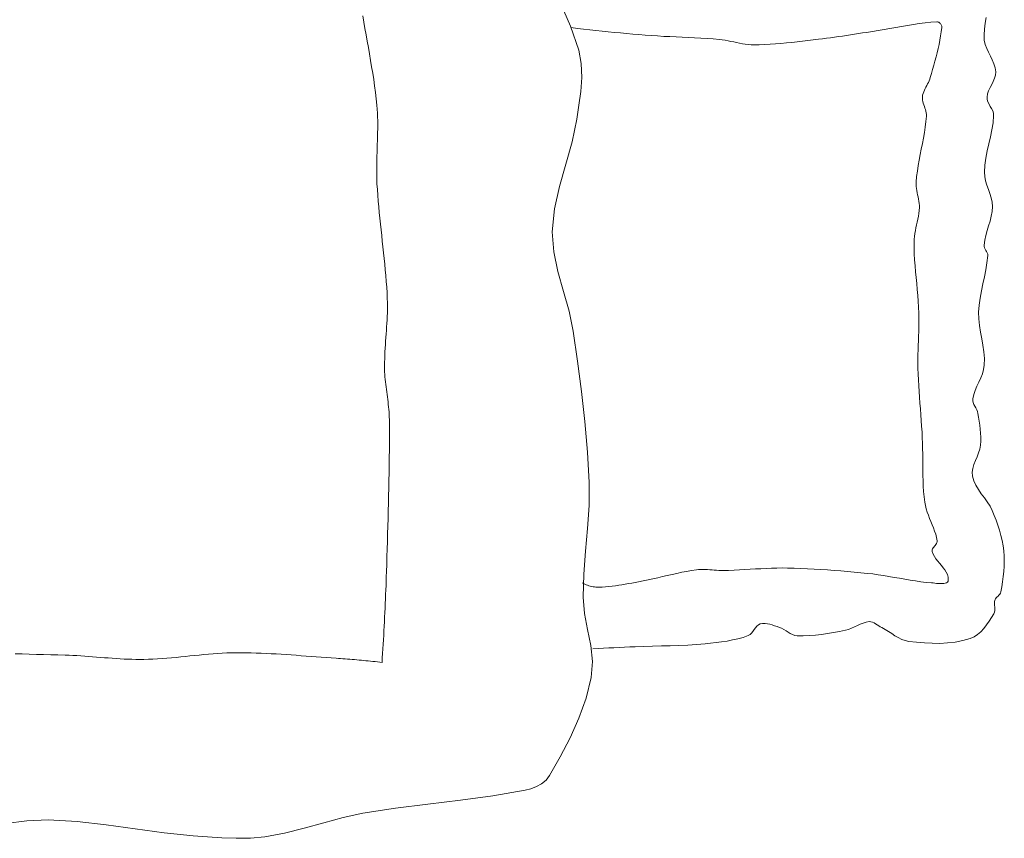
# Model space of a CAD drawing. Units: inches. Extents: x -36302355 to 648, y -221479757 to 75.
# Tile 18 of 37: x 555 to 590, y -530 to -501. Entities that reach past the tile are written whole.
import ezdxf

# ---------------------------------------------------------------- set-up
doc = ezdxf.new("R2010")
doc.units = ezdxf.units.IN
doc.header["$MEASUREMENT"] = 0
doc.layers.add('A-FURN', color=8, linetype='Continuous', lineweight=13)

# ---------------------------------------------------------------- blocks, each defined once
blk = doc.blocks.new('BED-DOUBLE')
for p, q in [((46.094, 79.977), (45.912, 79.943)), ((46.276, 80.001), (46.094, 79.977)), ((46.457, 80.015), (46.276, 80.001)), ((46.638, 80.019), (46.457, 80.015)), ((46.819, 80.013), (46.638, 80.019)), ((47.001, 80.001), (46.819, 80.013)), ((47.182, 79.981), (47.001, 80.001)), ((47.363, 79.957), (47.182, 79.981)), ((29.156, 79.653), (29.019, 79.595)), ((29.295, 79.695), (29.156, 79.653)), ((29.439, 79.716), (29.295, 79.695)), ((29.555, 79.707), (29.439, 79.716)), ((29.667, 79.676), (29.555, 79.707)), ((29.776, 79.63), (29.667, 79.676)), ((29.885, 79.575), (29.776, 79.63)), ((30.892, 79.636), (30.811, 79.61)), ((30.976, 79.644), (30.892, 79.636)), ((31.228, 79.624), (30.976, 79.644)), ((31.477, 79.585), (31.228, 79.624)), ((45.03, 79.665), (44.859, 79.595)), ((45.203, 79.731), (45.03, 79.665)), ((45.378, 79.793), (45.203, 79.731)), ((45.554, 79.85), (45.378, 79.793)), ((45.733, 79.9), (45.554, 79.85)), ((45.912, 79.943), (45.733, 79.9)), ((47.542, 79.928), (47.363, 79.957)), ((47.721, 79.897), (47.542, 79.928)), ((47.762, 79.883), (47.721, 79.897)), ((47.799, 79.86), (47.762, 79.883)), ((47.832, 79.831), (47.799, 79.86)), ((47.865, 79.797), (47.832, 79.831)), ((47.897, 79.763), (47.865, 79.797)), ((47.93, 79.732), (47.897, 79.763)), ((47.966, 79.705), (47.93, 79.732)), ((48.005, 79.687), (47.966, 79.705)), ((48.065, 79.675), (48.005, 79.687)), ((48.126, 79.673), (48.065, 79.675)), ((48.189, 79.677), (48.126, 79.673)), ((48.253, 79.684), (48.189, 79.677)), ((48.316, 79.688), (48.253, 79.684)), ((48.376, 79.687), (48.316, 79.688)), ((48.434, 79.676), (48.376, 79.687)), ((48.487, 79.652), (48.434, 79.676)), ((48.617, 79.57), (48.487, 79.652)), ((27.733, 79.348), (27.532, 79.381)), ((27.935, 79.319), (27.733, 79.348)), ((28.135, 79.305), (27.935, 79.319)), ((28.332, 79.316), (28.135, 79.305)), ((28.475, 79.348), (28.332, 79.316)), ((28.614, 79.399), (28.475, 79.348)), ((28.75, 79.461), (28.614, 79.399)), ((28.885, 79.529), (28.75, 79.461)), ((29.019, 79.595), (28.885, 79.529)), ((29.994, 79.518), (29.885, 79.575)), ((30.103, 79.467), (29.994, 79.518)), ((30.215, 79.429), (30.103, 79.467)), ((30.331, 79.412), (30.215, 79.429)), ((30.415, 79.419), (30.331, 79.412)), ((30.496, 79.445), (30.415, 79.419)), ((30.575, 79.483), (30.496, 79.445)), ((30.654, 79.527), (30.575, 79.483)), ((30.732, 79.571), (30.654, 79.527)), ((30.811, 79.61), (30.732, 79.571)), ((31.725, 79.534), (31.477, 79.585)), ((31.973, 79.478), (31.725, 79.534)), ((32.221, 79.421), (31.973, 79.478)), ((32.469, 79.372), (32.221, 79.421)), ((32.718, 79.336), (32.469, 79.372)), ((32.97, 79.321), (32.718, 79.336)), ((33.123, 79.331), (32.97, 79.321)), ((33.273, 79.362), (33.123, 79.331)), ((33.423, 79.406), (33.273, 79.362)), ((33.571, 79.458), (33.423, 79.406)), ((33.72, 79.51), (33.571, 79.458)), ((33.869, 79.555), (33.72, 79.51)), ((34.02, 79.587), (33.869, 79.555)), ((34.173, 79.598), (34.02, 79.587)), ((34.345, 79.587), (34.173, 79.598)), ((34.515, 79.557), (34.345, 79.587)), ((34.684, 79.516), (34.515, 79.557)), ((34.852, 79.467), (34.684, 79.516)), ((35.02, 79.416), (34.852, 79.467)), ((35.188, 79.369), (35.02, 79.416)), ((35.358, 79.33), (35.188, 79.369)), ((35.529, 79.305), (35.358, 79.33)), ((35.577, 79.308), (35.529, 79.305)), ((35.623, 79.323), (35.577, 79.308)), ((35.669, 79.345), (35.623, 79.323)), ((35.714, 79.371), (35.669, 79.345)), ((35.758, 79.398), (35.714, 79.371)), ((35.804, 79.42), (35.758, 79.398)), ((35.85, 79.435), (35.804, 79.42)), ((35.898, 79.439), (35.85, 79.435)), ((36.149, 79.41), (35.898, 79.439)), ((36.398, 79.368), (36.149, 79.41)), ((36.646, 79.318), (36.398, 79.368)), ((36.894, 79.264), (36.646, 79.318)), ((39.283, 79.299), (39.051, 79.265)), ((39.515, 79.318), (39.283, 79.299)), ((39.748, 79.315), (39.515, 79.318)), ((39.902, 79.292), (39.748, 79.315)), ((40.051, 79.248), (39.902, 79.292)), ((44.409, 79.317), (44.266, 79.21)), ((44.554, 79.421), (44.409, 79.317)), ((44.703, 79.516), (44.554, 79.421)), ((44.859, 79.595), (44.703, 79.516)), ((48.749, 79.484), (48.617, 79.57)), ((48.879, 79.394), (48.749, 79.484)), ((49.004, 79.298), (48.879, 79.394)), ((49.119, 79.194), (49.004, 79.298)), ((37.142, 79.212), (36.894, 79.264)), ((37.39, 79.167), (37.142, 79.212)), ((37.64, 79.133), (37.39, 79.167)), ((37.891, 79.115), (37.64, 79.133)), ((38.124, 79.119), (37.891, 79.115)), ((38.357, 79.144), (38.124, 79.119)), ((38.588, 79.18), (38.357, 79.144)), ((38.82, 79.223), (38.588, 79.18)), ((39.051, 79.265), (38.82, 79.223)), ((40.198, 79.189), (40.051, 79.248)), ((40.343, 79.122), (40.198, 79.189)), ((40.488, 79.055), (40.343, 79.122)), ((40.634, 78.992), (40.488, 79.055)), ((40.783, 78.942), (40.634, 78.992)), ((40.936, 78.91), (40.783, 78.942)), ((41.066, 78.924), (41.002, 78.91)), ((41.128, 78.95), (41.066, 78.924)), ((41.19, 78.981), (41.128, 78.95)), ((41.252, 79.016), (41.19, 78.981)), ((41.315, 79.048), (41.252, 79.016)), ((41.378, 79.075), (41.315, 79.048)), ((41.444, 79.093), (41.378, 79.075)), ((41.582, 79.116), (41.444, 79.093)), ((41.721, 79.137), (41.582, 79.116)), ((41.86, 79.157), (41.721, 79.137)), ((42, 79.173), (41.86, 79.157)), ((42.139, 79.184), (42, 79.173)), ((42.279, 79.19), (42.139, 79.184)), ((42.419, 79.19), (42.279, 79.19)), ((42.558, 79.182), (42.419, 79.19)), ((42.698, 79.158), (42.558, 79.182)), ((42.835, 79.114), (42.698, 79.158)), ((42.971, 79.06), (42.835, 79.114)), ((43.106, 79.003), (42.971, 79.06)), ((43.241, 78.95), (43.106, 79.003)), ((43.377, 78.91), (43.241, 78.95)), ((43.817, 78.944), (43.651, 78.898)), ((43.972, 79.016), (43.817, 78.944)), ((44.121, 79.107), (43.972, 79.016)), ((44.266, 79.21), (44.121, 79.107)), ((49.219, 79.081), (49.119, 79.194)), ((49.301, 78.957), (49.219, 79.081)), ((49.36, 78.82), (49.301, 78.957)), ((41.002, 78.91), (40.936, 78.91)), ((43.513, 78.89), (43.377, 78.91)), ((43.651, 78.898), (43.513, 78.89)), ((49.432, 78.561), (49.36, 78.82)), ((49.482, 78.296), (49.432, 78.561)), ((49.513, 78.027), (49.482, 78.296)), ((46.868, 77.87), (46.947, 77.928)), ((46.947, 77.928), (47.028, 77.978)), ((47.028, 77.978), (47.112, 78.016)), ((47.112, 78.016), (47.2, 78.041)), ((47.2, 78.041), (47.293, 78.049)), ((47.293, 78.049), (47.337, 78.04)), ((47.337, 78.04), (47.371, 78.018)), ((47.371, 78.018), (47.396, 77.983)), ((47.396, 77.983), (47.413, 77.939)), ((47.413, 77.939), (47.423, 77.887)), ((47.423, 77.887), (47.427, 77.828)), ((49.527, 77.755), (49.513, 78.027)), ((27.683, 77.649), (27.684, 77.671)), ((27.699, 77.441), (27.683, 77.649)), ((27.684, 77.671), (27.689, 77.693)), ((27.689, 77.693), (27.699, 77.715)), ((27.699, 77.715), (27.712, 77.735)), ((27.712, 77.735), (27.728, 77.755)), ((27.728, 77.755), (27.746, 77.773)), ((27.746, 77.773), (27.767, 77.789)), ((27.767, 77.789), (27.789, 77.803)), ((27.789, 77.803), (27.812, 77.813)), ((27.812, 77.813), (27.835, 77.821)), ((27.835, 77.821), (27.858, 77.824)), ((27.858, 77.824), (27.88, 77.824)), ((27.88, 77.824), (28.029, 77.804)), ((28.029, 77.804), (28.178, 77.781)), ((28.178, 77.781), (28.326, 77.754)), ((28.326, 77.754), (28.474, 77.723)), ((28.474, 77.723), (28.621, 77.691)), ((28.621, 77.691), (28.768, 77.655)), ((28.768, 77.655), (28.915, 77.618)), ((28.915, 77.618), (29.061, 77.58)), ((29.061, 77.58), (29.206, 77.54)), ((29.206, 77.54), (29.352, 77.499)), ((45.467, 77.529), (45.579, 77.57)), ((45.579, 77.57), (45.692, 77.607)), ((45.692, 77.607), (45.806, 77.636)), ((45.806, 77.636), (45.922, 77.659)), ((45.922, 77.659), (45.956, 77.659)), ((45.956, 77.659), (45.988, 77.65)), ((45.988, 77.65), (46.02, 77.634)), ((46.02, 77.634), (46.051, 77.613)), ((46.051, 77.613), (46.082, 77.589)), ((46.082, 77.589), (46.112, 77.564)), ((46.112, 77.564), (46.142, 77.538)), ((46.142, 77.538), (46.172, 77.515)), ((46.388, 77.515), (46.473, 77.56)), ((46.473, 77.56), (46.555, 77.615)), ((46.555, 77.615), (46.635, 77.677)), ((46.635, 77.677), (46.713, 77.741)), ((46.713, 77.741), (46.79, 77.807)), ((46.79, 77.807), (46.868, 77.87)), ((47.412, 77.574), (47.405, 77.515)), ((47.418, 77.637), (47.412, 77.574)), ((47.424, 77.701), (47.418, 77.637)), ((47.427, 77.766), (47.424, 77.701)), ((47.427, 77.828), (47.427, 77.766)), ((49.526, 77.481), (49.527, 77.755)), ((27.721, 77.234), (27.699, 77.441)), ((27.746, 77.027), (27.721, 77.234)), ((29.352, 77.499), (29.497, 77.458)), ((29.497, 77.458), (29.643, 77.417)), ((29.643, 77.417), (29.7, 77.398)), ((29.7, 77.398), (29.757, 77.376)), ((29.757, 77.376), (29.813, 77.349)), ((29.813, 77.349), (29.867, 77.321)), ((29.867, 77.321), (29.922, 77.292)), ((29.922, 77.292), (29.977, 77.263)), ((29.977, 77.263), (30.031, 77.234)), ((30.031, 77.234), (30.086, 77.207)), ((30.086, 77.207), (30.142, 77.184)), ((30.599, 77.187), (30.656, 77.207)), ((30.656, 77.207), (30.712, 77.227)), ((30.712, 77.227), (30.768, 77.246)), ((30.768, 77.246), (30.824, 77.261)), ((30.824, 77.261), (30.881, 77.273)), ((30.881, 77.273), (30.938, 77.28)), ((30.938, 77.28), (30.995, 77.28)), ((30.995, 77.28), (31.19, 77.261)), ((31.19, 77.261), (31.384, 77.237)), ((31.384, 77.237), (31.577, 77.207)), ((31.577, 77.207), (31.77, 77.173)), ((44.193, 77.181), (44.381, 77.199)), ((44.381, 77.199), (44.568, 77.222)), ((44.568, 77.222), (44.684, 77.244)), ((44.684, 77.244), (44.799, 77.273)), ((44.799, 77.273), (44.912, 77.309)), ((44.912, 77.309), (45.023, 77.35)), ((45.023, 77.35), (45.135, 77.394)), ((45.135, 77.394), (45.245, 77.439)), ((45.245, 77.439), (45.356, 77.485)), ((45.356, 77.485), (45.467, 77.529)), ((46.172, 77.515), (46.203, 77.496)), ((46.203, 77.496), (46.234, 77.483)), ((46.234, 77.483), (46.266, 77.478)), ((46.266, 77.478), (46.299, 77.482)), ((46.299, 77.482), (46.388, 77.515)), ((47.383, 77.273), (47.36, 77.084)), ((47.4, 77.462), (47.383, 77.273)), ((47.405, 77.515), (47.4, 77.462)), ((49.49, 76.936), (49.513, 77.208)), ((49.513, 77.208), (49.526, 77.481)), ((27.776, 76.821), (27.746, 77.027)), ((30.142, 77.184), (30.199, 77.164)), ((30.199, 77.164), (30.257, 77.148)), ((30.257, 77.148), (30.316, 77.139)), ((30.316, 77.139), (30.374, 77.137)), ((30.374, 77.137), (30.43, 77.142)), ((30.43, 77.142), (30.487, 77.153)), ((30.487, 77.153), (30.543, 77.169)), ((30.543, 77.169), (30.599, 77.187)), ((31.77, 77.173), (31.963, 77.137)), ((31.963, 77.137), (32.155, 77.099)), ((32.155, 77.099), (32.348, 77.062)), ((32.348, 77.062), (32.54, 77.025)), ((32.54, 77.025), (32.733, 76.991)), ((32.733, 76.991), (32.927, 76.961)), ((32.927, 76.961), (33.12, 76.936)), ((33.12, 76.936), (33.315, 76.917)), ((33.315, 76.917), (33.39, 76.915)), ((33.39, 76.915), (33.465, 76.919)), ((33.465, 76.919), (33.54, 76.927)), ((33.54, 76.927), (33.614, 76.939)), ((33.614, 76.939), (33.689, 76.954)), ((33.689, 76.954), (33.763, 76.97)), ((33.763, 76.97), (33.838, 76.986)), ((33.838, 76.986), (33.912, 77.002)), ((33.912, 77.002), (33.987, 77.015)), ((33.987, 77.015), (34.062, 77.026)), ((34.062, 77.026), (34.137, 77.032)), ((34.137, 77.032), (34.212, 77.032)), ((34.212, 77.032), (34.314, 77.026)), ((34.314, 77.026), (34.416, 77.014)), ((34.416, 77.014), (34.517, 76.997)), ((34.517, 76.997), (34.618, 76.978)), ((34.618, 76.978), (34.718, 76.956)), ((34.718, 76.956), (34.819, 76.934)), ((34.819, 76.934), (34.92, 76.912)), ((34.92, 76.912), (35.02, 76.891)), ((35.02, 76.891), (35.121, 76.873)), ((35.121, 76.873), (35.223, 76.858)), ((35.223, 76.858), (35.324, 76.848)), ((35.324, 76.848), (35.426, 76.845)), ((35.426, 76.845), (35.634, 76.847)), ((35.634, 76.847), (35.842, 76.854)), ((35.842, 76.854), (36.05, 76.866)), ((36.05, 76.866), (36.258, 76.881)), ((36.258, 76.881), (36.465, 76.899)), ((36.465, 76.899), (36.673, 76.918)), ((36.673, 76.918), (36.88, 76.938)), ((36.88, 76.938), (37.088, 76.957)), ((37.088, 76.957), (37.296, 76.976)), ((37.296, 76.976), (37.503, 76.992)), ((37.503, 76.992), (37.711, 77.005)), ((37.711, 77.005), (37.919, 77.014)), ((37.919, 77.014), (38.081, 77.017)), ((38.081, 77.017), (38.242, 77.017)), ((38.242, 77.017), (38.404, 77.015)), ((38.404, 77.015), (38.566, 77.011)), ((38.566, 77.011), (38.727, 77.006)), ((38.727, 77.006), (38.889, 77)), ((38.889, 77), (39.051, 76.993)), ((39.051, 76.993), (39.212, 76.988)), ((39.212, 76.988), (39.374, 76.984)), ((39.374, 76.984), (39.536, 76.981)), ((39.536, 76.981), (39.697, 76.981)), ((39.697, 76.981), (39.859, 76.984)), ((39.859, 76.984), (40.063, 76.991)), ((40.063, 76.991), (40.267, 77)), ((40.267, 77), (40.471, 77.011)), ((40.471, 77.011), (40.675, 77.024)), ((40.675, 77.024), (40.879, 77.038)), ((40.879, 77.038), (41.082, 77.053)), ((41.082, 77.053), (41.286, 77.068)), ((41.286, 77.068), (41.49, 77.083)), ((41.49, 77.083), (41.694, 77.098)), ((41.694, 77.098), (41.898, 77.112)), ((41.898, 77.112), (42.102, 77.125)), ((42.102, 77.125), (42.306, 77.136)), ((42.306, 77.136), (42.494, 77.144)), ((42.494, 77.144), (42.683, 77.148)), ((42.683, 77.148), (42.872, 77.151)), ((42.872, 77.151), (43.061, 77.152)), ((43.061, 77.152), (43.25, 77.152)), ((43.25, 77.152), (43.439, 77.153)), ((43.439, 77.153), (43.628, 77.156)), ((43.628, 77.156), (43.817, 77.161)), ((43.817, 77.161), (44.005, 77.169)), ((44.005, 77.169), (44.193, 77.181)), ((47.334, 76.896), (47.305, 76.708)), ((47.36, 77.084), (47.334, 76.896)), ((49.459, 76.667), (49.49, 76.936)), ((27.808, 76.615), (27.776, 76.821)), ((27.843, 76.41), (27.808, 76.615)), ((47.273, 76.52), (47.241, 76.333)), ((47.305, 76.708), (47.273, 76.52)), ((49.387, 76.412), (49.432, 76.537)), ((49.432, 76.537), (49.459, 76.667)), ((27.879, 76.204), (27.843, 76.41)), ((27.915, 75.999), (27.879, 76.204)), ((47.241, 76.333), (47.208, 76.145)), ((49.184, 76.059), (49.258, 76.175)), ((49.258, 76.175), (49.327, 76.292)), ((49.327, 76.292), (49.387, 76.412)), ((27.952, 75.793), (27.915, 75.999)), ((47.175, 75.958), (47.144, 75.77)), ((47.208, 76.145), (47.175, 75.958)), ((48.971, 75.709), (49.036, 75.827)), ((49.036, 75.827), (49.108, 75.944)), ((49.108, 75.944), (49.184, 76.059)), ((27.987, 75.588), (27.952, 75.793)), ((28.021, 75.382), (27.987, 75.588)), ((47.115, 75.582), (47.089, 75.394)), ((47.144, 75.77), (47.115, 75.582)), ((48.806, 75.441), (48.836, 75.495)), ((48.836, 75.495), (48.871, 75.549)), ((48.871, 75.549), (48.907, 75.602)), ((48.907, 75.602), (48.941, 75.655)), ((48.941, 75.655), (48.971, 75.709)), ((28.053, 75.176), (28.021, 75.382)), ((28.074, 75.036), (28.053, 75.176)), ((47.068, 75.205), (47.044, 74.972)), ((47.089, 75.394), (47.068, 75.205)), ((48.764, 75.269), (48.767, 75.329)), ((48.781, 75.161), (48.764, 75.269)), ((48.767, 75.329), (48.782, 75.386)), ((48.812, 75.056), (48.781, 75.161)), ((48.782, 75.386), (48.806, 75.441)), ((28.095, 74.896), (28.074, 75.036)), ((28.117, 74.755), (28.095, 74.896)), ((47.044, 74.972), (47.022, 74.739)), ((48.854, 74.954), (48.812, 75.056)), ((48.901, 74.853), (48.854, 74.954)), ((48.95, 74.751), (48.901, 74.853)), ((28.139, 74.615), (28.117, 74.755)), ((28.161, 74.475), (28.139, 74.615)), ((28.182, 74.335), (28.161, 74.475)), ((47.001, 74.505), (46.981, 74.272)), ((47.022, 74.739), (47.001, 74.505)), ((48.996, 74.649), (48.95, 74.751)), ((49.036, 74.546), (48.996, 74.649)), ((49.064, 74.439), (49.036, 74.546)), ((49.105, 74.229), (49.064, 74.439)), ((28.203, 74.194), (28.182, 74.335)), ((28.224, 74.054), (28.203, 74.194)), ((46.981, 74.272), (46.962, 74.038)), ((49.144, 74.017), (49.105, 74.229)), ((28.243, 73.914), (28.224, 74.054)), ((28.262, 73.773), (28.243, 73.914)), ((28.279, 73.632), (28.262, 73.773)), ((46.945, 73.805), (46.929, 73.571)), ((46.962, 74.038), (46.945, 73.805)), ((49.181, 73.805), (49.144, 74.017)), ((49.212, 73.592), (49.181, 73.805)), ((28.296, 73.491), (28.279, 73.632)), ((28.317, 73.302), (28.296, 73.491)), ((46.929, 73.571), (46.916, 73.337)), ((49.238, 73.379), (49.212, 73.592)), ((28.339, 73.113), (28.317, 73.302)), ((28.361, 72.924), (28.339, 73.113)), ((46.904, 73.103), (46.894, 72.869)), ((46.916, 73.337), (46.904, 73.103)), ((49.255, 73.166), (49.238, 73.379)), ((49.263, 72.952), (49.255, 73.166)), ((28.383, 72.734), (28.361, 72.924)), ((28.404, 72.545), (28.383, 72.734)), ((46.894, 72.869), (46.886, 72.635)), ((49.248, 72.654), (49.26, 72.738)), ((49.26, 72.738), (49.263, 72.952)), ((28.424, 72.356), (28.404, 72.545)), ((28.442, 72.166), (28.424, 72.356)), ((46.88, 72.401), (46.878, 72.212)), ((46.886, 72.635), (46.88, 72.401)), ((49.04, 72.269), (49.087, 72.345)), ((49.087, 72.345), (49.136, 72.42)), ((49.136, 72.42), (49.181, 72.496)), ((49.181, 72.496), (49.22, 72.573)), ((49.22, 72.573), (49.248, 72.654)), ((28.458, 71.976), (28.442, 72.166)), ((46.878, 72.212), (46.88, 72.024)), ((46.88, 72.024), (46.885, 71.835)), ((48.909, 71.945), (48.938, 72.028)), ((48.938, 72.028), (48.965, 72.11)), ((48.965, 72.11), (48.998, 72.191)), ((48.998, 72.191), (49.04, 72.269)), ((28.471, 71.786), (28.458, 71.976)), ((28.482, 71.596), (28.471, 71.786)), ((46.885, 71.835), (46.892, 71.647)), ((48.827, 71.607), (48.837, 71.692)), ((48.837, 71.692), (48.856, 71.777)), ((48.856, 71.777), (48.88, 71.861)), ((48.88, 71.861), (48.909, 71.945)), ((28.488, 71.406), (28.482, 71.596)), ((28.491, 71.216), (28.488, 71.406)), ((46.892, 71.647), (46.902, 71.458)), ((46.902, 71.458), (46.912, 71.27)), ((48.828, 71.523), (48.827, 71.607)), ((48.842, 71.44), (48.828, 71.523)), ((48.872, 71.375), (48.842, 71.44)), ((48.919, 71.32), (48.872, 71.375)), ((48.978, 71.271), (48.919, 71.32)), ((28.467, 70.911), (28.48, 71.012)), ((28.48, 71.012), (28.488, 71.114)), ((28.488, 71.114), (28.491, 71.216)), ((46.912, 71.27), (46.923, 71.081)), ((46.923, 71.081), (46.934, 70.893)), ((49.043, 71.226), (48.978, 71.271)), ((49.109, 71.182), (49.043, 71.226)), ((49.17, 71.134), (49.109, 71.182)), ((49.221, 71.08), (49.17, 71.134)), ((49.256, 71.016), (49.221, 71.08)), ((49.316, 70.833), (49.256, 71.016)), ((28.411, 70.608), (28.432, 70.709)), ((28.432, 70.709), (28.451, 70.81)), ((28.451, 70.81), (28.467, 70.911)), ((46.934, 70.893), (46.944, 70.704)), ((46.944, 70.704), (46.954, 70.516)), ((49.367, 70.648), (49.316, 70.833)), ((49.409, 70.46), (49.367, 70.648)), ((28.33, 70.205), (28.348, 70.306)), ((28.348, 70.306), (28.368, 70.407)), ((28.368, 70.407), (28.389, 70.508)), ((28.389, 70.508), (28.411, 70.608)), ((46.954, 70.516), (46.961, 70.327)), ((46.961, 70.327), (46.966, 70.138)), ((49.445, 70.27), (49.409, 70.46)), ((49.474, 70.079), (49.445, 70.27)), ((28.285, 69.785), (28.303, 70.002)), ((28.303, 70.002), (28.315, 70.104)), ((28.315, 70.104), (28.33, 70.205)), ((46.964, 69.98), (46.959, 69.901)), ((46.966, 70.059), (46.964, 69.98)), ((46.966, 70.138), (46.966, 70.059)), ((49.499, 69.887), (49.474, 70.079)), ((28.27, 69.568), (28.285, 69.785)), ((46.936, 69.585), (46.932, 69.506)), ((46.941, 69.664), (46.936, 69.585)), ((46.947, 69.743), (46.941, 69.664)), ((46.954, 69.822), (46.947, 69.743)), ((46.959, 69.901), (46.954, 69.822)), ((49.521, 69.695), (49.499, 69.887)), ((49.541, 69.503), (49.521, 69.695)), ((28.244, 69.133), (28.256, 69.35)), ((28.256, 69.35), (28.27, 69.568)), ((46.932, 69.506), (46.93, 69.427)), ((46.93, 69.427), (46.93, 69.349)), ((46.93, 69.349), (46.934, 69.27)), ((46.934, 69.27), (46.943, 69.192)), ((49.567, 69.196), (49.541, 69.503)), ((28.223, 68.697), (28.234, 68.915)), ((28.234, 68.915), (28.244, 69.133)), ((46.943, 69.192), (46.968, 69.02)), ((46.968, 69.02), (46.997, 68.85)), ((49.586, 68.889), (49.567, 69.196)), ((49.6, 68.581), (49.586, 68.889)), ((28.213, 68.48), (28.223, 68.697)), ((46.997, 68.85), (47.03, 68.679)), ((47.03, 68.679), (47.066, 68.51)), ((49.611, 68.273), (49.6, 68.581)), ((28.192, 68.045), (28.203, 68.262)), ((28.203, 68.262), (28.213, 68.48)), ((47.066, 68.51), (47.103, 68.34)), ((47.103, 68.34), (47.142, 68.171)), ((49.619, 67.964), (49.611, 68.273)), ((28.18, 67.827), (28.192, 68.045)), ((47.142, 68.171), (47.182, 68.002)), ((47.182, 68.002), (47.221, 67.833)), ((49.627, 67.656), (49.619, 67.964)), ((28.15, 67.392), (28.166, 67.61)), ((28.166, 67.61), (28.18, 67.827)), ((47.221, 67.833), (47.26, 67.664)), ((47.26, 67.664), (47.297, 67.495)), ((49.636, 67.348), (49.627, 67.656)), ((28.113, 66.959), (28.132, 67.176)), ((28.132, 67.176), (28.15, 67.392)), ((47.297, 67.495), (47.332, 67.325)), ((47.332, 67.325), (47.364, 67.155)), ((47.364, 67.155), (47.385, 67.039)), ((49.647, 67.04), (49.636, 67.348)), ((28.094, 66.742), (28.113, 66.959)), ((47.385, 67.039), (47.406, 66.924)), ((47.406, 66.924), (47.428, 66.809)), ((47.428, 66.809), (47.448, 66.693)), ((49.655, 66.854), (49.647, 67.04)), ((49.664, 66.668), (49.655, 66.854)), ((28.053, 66.309), (28.074, 66.526)), ((28.074, 66.526), (28.094, 66.742)), ((47.448, 66.693), (47.468, 66.577)), ((47.468, 66.577), (47.487, 66.462)), ((47.487, 66.462), (47.504, 66.346)), ((49.672, 66.482), (49.664, 66.668)), ((49.68, 66.296), (49.672, 66.482)), ((28.032, 66.093), (28.053, 66.309)), ((47.504, 66.346), (47.519, 66.23)), ((47.519, 66.23), (47.532, 66.113)), ((47.532, 66.113), (47.543, 65.997)), ((49.689, 66.11), (49.68, 66.296)), ((27.987, 65.66), (28.01, 65.876)), ((28.01, 65.876), (28.032, 66.093)), ((47.543, 65.997), (47.55, 65.88)), ((47.55, 65.88), (47.554, 65.763)), ((49.697, 65.924), (49.689, 66.11)), ((49.706, 65.738), (49.697, 65.924)), ((27.938, 65.228), (27.963, 65.444)), ((27.963, 65.444), (27.987, 65.66)), ((43.87, 65.425), (42.802, 65.366)), ((44.678, 65.422), (43.87, 65.425)), ((45.485, 65.369), (44.678, 65.422)), ((47.515, 65.464), (47.501, 65.415)), ((47.527, 65.513), (47.515, 65.464)), ((47.537, 65.563), (47.527, 65.513)), ((47.545, 65.613), (47.537, 65.563)), ((47.55, 65.663), (47.545, 65.613)), ((47.553, 65.713), (47.55, 65.663)), ((47.554, 65.763), (47.553, 65.713)), ((49.604, 65.477), (49.04, 65.369)), ((50.166, 65.538), (49.604, 65.477)), ((49.715, 65.552), (49.706, 65.738)), ((50.724, 65.499), (50.166, 65.538)), ((51.45, 65.318), (50.724, 65.499)), ((27.913, 65.012), (27.938, 65.228)), ((29.152, 65.148), (28.68, 65.056)), ((29.636, 65.165), (29.152, 65.148)), ((30.126, 65.13), (29.636, 65.165)), ((30.616, 65.064), (30.126, 65.13)), ((40.671, 65.153), (39.609, 65.014)), ((41.735, 65.273), (40.671, 65.153)), ((42.802, 65.366), (41.735, 65.273)), ((46.292, 65.296), (45.485, 65.369)), ((47.1, 65.235), (46.292, 65.296)), ((47.908, 65.214), (47.1, 65.235)), ((47.422, 65.229), (47.397, 65.186)), ((47.445, 65.274), (47.422, 65.229)), ((47.466, 65.32), (47.445, 65.274)), ((47.484, 65.367), (47.466, 65.32)), ((47.501, 65.415), (47.484, 65.367)), ((48.474, 65.264), (47.908, 65.214)), ((49.04, 65.369), (48.474, 65.264)), ((52.158, 65.065), (51.45, 65.318)), ((27.839, 64.768), (27.022, 64.416)), ((28.68, 65.056), (27.839, 64.768)), ((27.887, 64.796), (27.913, 65.012)), ((31.101, 64.99), (30.616, 65.064)), ((31.896, 64.828), (31.101, 64.99)), ((32.683, 64.608), (31.896, 64.828)), ((38.549, 64.862), (37.849, 64.716)), ((39.609, 65.014), (38.549, 64.862)), ((52.846, 64.755), (52.158, 65.065)), ((53.517, 64.405), (52.846, 64.755)), ((33.469, 64.384), (32.683, 64.608)), ((34.259, 64.206), (33.469, 64.384)), ((37.155, 64.522), (36.463, 64.326)), ((37.849, 64.716), (37.155, 64.522)), ((54.172, 64.032), (53.517, 64.405)), ((35.061, 64.125), (34.259, 64.206)), ((35.767, 64.177), (35.061, 64.125)), ((36.463, 64.326), (35.767, 64.177)), ((54.33, 63.91), (54.172, 64.032)), ((54.459, 63.752), (54.33, 63.91)), ((54.561, 63.57), (54.459, 63.752)), ((54.638, 63.375), (54.561, 63.57)), ((54.689, 63.176), (54.638, 63.375)), ((54.886, 62.042), (54.689, 63.176)), ((55.039, 60.9), (54.886, 62.042)), ((55.175, 59.755), (55.039, 60.9)), ((55.318, 58.611), (55.175, 59.755)), ((55.495, 57.473), (55.318, 58.611)), ((35.393, 58.153), (35.191, 58.131)), ((35.594, 58.175), (35.393, 58.153)), ((35.796, 58.197), (35.594, 58.175)), ((35.998, 58.218), (35.796, 58.197)), ((36.2, 58.239), (35.998, 58.218)), ((36.401, 58.258), (36.2, 58.239)), ((36.603, 58.276), (36.401, 58.258)), ((36.806, 58.292), (36.603, 58.276)), ((37.008, 58.306), (36.806, 58.292)), ((37.21, 58.318), (37.008, 58.306)), ((37.413, 58.327), (37.21, 58.318)), ((37.537, 58.331), (37.413, 58.327)), ((37.661, 58.333), (37.537, 58.331)), ((37.785, 58.332), (37.661, 58.333)), ((37.909, 58.329), (37.785, 58.332)), ((38.034, 58.325), (37.909, 58.329)), ((38.158, 58.319), (38.034, 58.325)), ((38.282, 58.313), (38.158, 58.319)), ((38.406, 58.305), (38.282, 58.313)), ((38.53, 58.296), (38.406, 58.305)), ((38.654, 58.288), (38.53, 58.296)), ((38.779, 58.279), (38.654, 58.288)), ((38.903, 58.27), (38.779, 58.279)), ((39.027, 58.261), (38.903, 58.27)), ((39.151, 58.253), (39.027, 58.261)), ((39.275, 58.246), (39.151, 58.253)), ((39.4, 58.241), (39.275, 58.246)), ((39.524, 58.236), (39.4, 58.241)), ((39.648, 58.233), (39.524, 58.236)), ((39.772, 58.232), (39.648, 58.233)), ((39.896, 58.233), (39.772, 58.232)), ((39.985, 58.235), (39.896, 58.233)), ((40.073, 58.24), (39.985, 58.235)), ((40.162, 58.246), (40.073, 58.24)), ((40.25, 58.254), (40.162, 58.246)), ((40.338, 58.262), (40.25, 58.254)), ((40.426, 58.272), (40.338, 58.262)), ((40.514, 58.283), (40.426, 58.272)), ((40.603, 58.294), (40.514, 58.283)), ((40.691, 58.306), (40.603, 58.294)), ((40.779, 58.318), (40.691, 58.306)), ((40.867, 58.33), (40.779, 58.318)), ((40.955, 58.342), (40.867, 58.33)), ((41.043, 58.353), (40.955, 58.342)), ((41.131, 58.363), (41.043, 58.353)), ((41.219, 58.373), (41.131, 58.363)), ((41.307, 58.381), (41.219, 58.373)), ((41.395, 58.389), (41.307, 58.381)), ((41.484, 58.394), (41.395, 58.389)), ((41.572, 58.398), (41.484, 58.394)), ((41.661, 58.4), (41.572, 58.398)), ((41.928, 58.402), (41.661, 58.4)), ((42.196, 58.402), (41.928, 58.402)), ((42.464, 58.402), (42.196, 58.402)), ((42.731, 58.401), (42.464, 58.402)), ((42.999, 58.398), (42.731, 58.401)), ((43.267, 58.395), (42.999, 58.398)), ((43.535, 58.391), (43.267, 58.395)), ((43.802, 58.386), (43.535, 58.391)), ((44.07, 58.381), (43.802, 58.386)), ((44.338, 58.375), (44.07, 58.381)), ((44.605, 58.368), (44.338, 58.375)), ((44.873, 58.362), (44.605, 58.368)), ((45.141, 58.354), (44.873, 58.362)), ((45.408, 58.346), (45.141, 58.354)), ((45.676, 58.339), (45.408, 58.346)), ((45.944, 58.33), (45.676, 58.339)), ((46.211, 58.322), (45.944, 58.33)), ((46.479, 58.314), (46.211, 58.322)), ((46.746, 58.306), (46.479, 58.314)), ((47.014, 58.298), (46.746, 58.306)), ((47.173, 58.293), (47.014, 58.298)), ((47.333, 58.287), (47.173, 58.293)), ((47.492, 58.282), (47.333, 58.287)), ((47.651, 58.276), (47.492, 58.282)), ((47.81, 58.27), (47.651, 58.276)), ((47.97, 58.263), (47.81, 58.27)), ((48.129, 58.257), (47.97, 58.263)), ((48.288, 58.25), (48.129, 58.257)), ((48.447, 58.242), (48.288, 58.25)), ((48.606, 58.235), (48.447, 58.242)), ((48.766, 58.227), (48.606, 58.235)), ((48.925, 58.219), (48.766, 58.227)), ((49.084, 58.21), (48.925, 58.219)), ((49.243, 58.201), (49.084, 58.21)), ((49.402, 58.192), (49.243, 58.201)), ((49.561, 58.183), (49.402, 58.192)), ((49.72, 58.173), (49.561, 58.183)), ((49.879, 58.163), (49.72, 58.173)), ((50.038, 58.153), (49.879, 58.163)), ((50.197, 58.142), (50.038, 58.153)), ((29.485, 57.815), (29.261, 57.778)), ((29.71, 57.849), (29.485, 57.815)), ((29.935, 57.881), (29.71, 57.849)), ((30.161, 57.91), (29.935, 57.881)), ((30.386, 57.937), (30.161, 57.91)), ((30.613, 57.96), (30.386, 57.937)), ((30.75, 57.972), (30.613, 57.96)), ((30.888, 57.98), (30.75, 57.972)), ((31.026, 57.986), (30.888, 57.98)), ((31.163, 57.989), (31.026, 57.986)), ((31.301, 57.991), (31.163, 57.989)), ((31.439, 57.99), (31.301, 57.991)), ((31.577, 57.988), (31.439, 57.99)), ((31.716, 57.985), (31.577, 57.988)), ((31.854, 57.981), (31.716, 57.985)), ((31.992, 57.977), (31.854, 57.981)), ((32.13, 57.972), (31.992, 57.977)), ((32.268, 57.967), (32.13, 57.972)), ((32.407, 57.963), (32.268, 57.967)), ((32.545, 57.959), (32.407, 57.963)), ((32.683, 57.956), (32.545, 57.959)), ((32.821, 57.954), (32.683, 57.956)), ((32.959, 57.954), (32.821, 57.954)), ((33.097, 57.956), (32.959, 57.954)), ((33.235, 57.959), (33.097, 57.956)), ((33.373, 57.965), (33.235, 57.959)), ((33.576, 57.978), (33.373, 57.965)), ((33.778, 57.992), (33.576, 57.978)), ((33.98, 58.008), (33.778, 57.992)), ((34.182, 58.026), (33.98, 58.008)), ((34.384, 58.045), (34.182, 58.026)), ((34.586, 58.065), (34.384, 58.045)), ((34.788, 58.087), (34.586, 58.065)), ((34.989, 58.108), (34.788, 58.087)), ((35.191, 58.131), (34.989, 58.108)), ((50.153, 57.739), (50.162, 57.82)), ((50.162, 57.82), (50.17, 57.9)), ((50.17, 57.9), (50.179, 57.981)), ((50.179, 57.981), (50.188, 58.062)), ((50.188, 58.062), (50.197, 58.142)), ((27.691, 57.503), (27.467, 57.465)), ((27.916, 57.542), (27.691, 57.503)), ((28.14, 57.582), (27.916, 57.542)), ((28.364, 57.622), (28.14, 57.582)), ((28.588, 57.662), (28.364, 57.622)), ((28.812, 57.702), (28.588, 57.662)), ((29.036, 57.741), (28.812, 57.702)), ((29.261, 57.778), (29.036, 57.741)), ((50.122, 57.416), (50.129, 57.497)), ((50.129, 57.497), (50.137, 57.577)), ((50.137, 57.577), (50.145, 57.658)), ((50.145, 57.658), (50.153, 57.739)), ((55.646, 56.779), (55.495, 57.473)), ((50.093, 57.092), (50.1, 57.173)), ((50.1, 57.173), (50.107, 57.254)), ((50.107, 57.254), (50.114, 57.335)), ((50.114, 57.335), (50.122, 57.416)), ((50.062, 56.688), (50.068, 56.769)), ((50.068, 56.769), (50.074, 56.85)), ((50.074, 56.85), (50.08, 56.931)), ((50.08, 56.931), (50.086, 57.012)), ((50.086, 57.012), (50.093, 57.092)), ((55.831, 56.091), (55.646, 56.779)), ((50.039, 56.35), (50.051, 56.526)), ((50.051, 56.526), (50.056, 56.607)), ((50.056, 56.607), (50.062, 56.688)), ((50.013, 56), (50.026, 56.175)), ((50.026, 56.175), (50.039, 56.35)), ((56.024, 55.406), (55.831, 56.091)), ((49.987, 55.649), (50, 55.824)), ((50, 55.824), (50.013, 56)), ((49.96, 55.298), (49.973, 55.474)), ((49.973, 55.474), (49.987, 55.649)), ((56.197, 54.717), (56.024, 55.406)), ((49.934, 54.947), (49.947, 55.123)), ((49.947, 55.123), (49.96, 55.298)), ((49.91, 54.596), (49.922, 54.772)), ((49.922, 54.772), (49.934, 54.947)), ((56.323, 54.019), (56.197, 54.717)), ((49.89, 54.245), (49.9, 54.421)), ((49.9, 54.421), (49.91, 54.596)), ((49.873, 53.894), (49.881, 54.07)), ((49.881, 54.07), (49.89, 54.245)), ((56.369, 53.519), (56.323, 54.019)), ((49.862, 53.543), (49.867, 53.719)), ((49.867, 53.719), (49.873, 53.894)), ((49.857, 53.192), (49.859, 53.367)), ((49.859, 53.367), (49.862, 53.543)), ((56.379, 53.016), (56.369, 53.519)), ((49.857, 53.016), (49.857, 53.192)), ((49.859, 52.853), (49.857, 53.016)), ((56.363, 52.512), (56.379, 53.016)), ((49.865, 52.69), (49.859, 52.853)), ((49.872, 52.527), (49.865, 52.69)), ((49.882, 52.365), (49.872, 52.527)), ((49.894, 52.202), (49.882, 52.365)), ((56.33, 52.008), (56.363, 52.512)), ((49.907, 52.04), (49.894, 52.202)), ((49.922, 51.877), (49.907, 52.04)), ((56.292, 51.505), (56.33, 52.008)), ((49.938, 51.715), (49.922, 51.877)), ((49.954, 51.553), (49.938, 51.715)), ((49.971, 51.39), (49.954, 51.553)), ((49.988, 51.228), (49.971, 51.39)), ((56.186, 50.484), (56.292, 51.505)), ((50.004, 51.065), (49.988, 51.228)), ((50.02, 50.903), (50.004, 51.065)), ((50.035, 50.741), (50.02, 50.903)), ((50.049, 50.578), (50.035, 50.741)), ((50.062, 50.416), (50.049, 50.578)), ((50.072, 50.253), (50.062, 50.416)), ((50.081, 50.09), (50.072, 50.253)), ((56.047, 49.466), (56.186, 50.484)), ((50.087, 49.927), (50.081, 50.09)), ((50.091, 49.764), (50.087, 49.927)), ((50.092, 49.626), (50.091, 49.764)), ((50.091, 49.488), (50.092, 49.626)), ((50.077, 49.073), (50.083, 49.211)), ((50.083, 49.211), (50.088, 49.349)), ((50.088, 49.349), (50.091, 49.488)), ((55.905, 48.448), (56.047, 49.466)), ((50.061, 48.797), (50.069, 48.935)), ((50.069, 48.935), (50.077, 49.073)), ((50.031, 48.382), (50.041, 48.52)), ((50.041, 48.52), (50.051, 48.658)), ((50.051, 48.658), (50.061, 48.797)), ((50.009, 48.106), (50.02, 48.244)), ((50.02, 48.244), (50.031, 48.382)), ((55.79, 47.428), (55.905, 48.448)), ((49.977, 47.691), (49.987, 47.83)), ((49.987, 47.83), (49.998, 47.968)), ((49.998, 47.968), (50.009, 48.106)), ((49.959, 47.415), (49.968, 47.553)), ((49.968, 47.553), (49.977, 47.691)), ((55.733, 46.404), (55.79, 47.428)), ((49.941, 47), (49.946, 47.138)), ((49.946, 47.138), (49.952, 47.277)), ((49.952, 47.277), (49.959, 47.415)), ((49.927, 46.497), (49.934, 46.749)), ((49.934, 46.749), (49.941, 47)), ((49.92, 46.246), (49.927, 46.497)), ((55.763, 45.66), (55.733, 46.404)), ((49.913, 45.995), (49.92, 46.246)), ((49.899, 45.492), (49.906, 45.743)), ((49.906, 45.743), (49.913, 45.995)), ((49.893, 45.241), (49.899, 45.492)), ((55.854, 44.918), (55.763, 45.66))]:
    blk.add_line(p, q)

msp = doc.modelspace()

# ---------------------------------------------------------------- block references
at = {"layer": 'A-FURN', "rotation": 270}
msp.add_blockref('BED-DOUBLE', (509.53, -473.482), dxfattribs=at)

doc.saveas('drawing.dxf')
